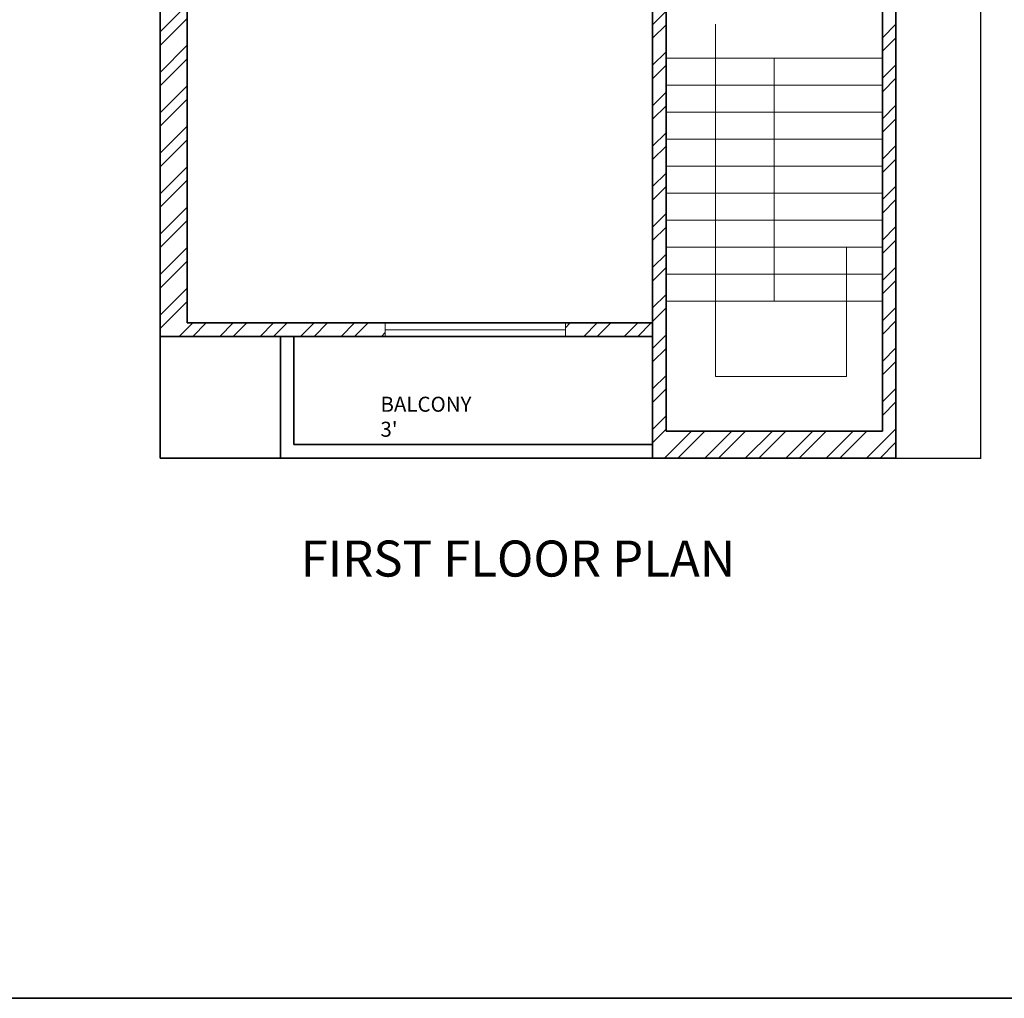
# Model space of a CAD drawing. Units: inches. Extents: x 1850 to 3445, y 1558 to 2756.
# Tile 5 of 13: x 2304 to 2632, y 1558 to 1884. Entities that reach past the tile are written whole.
import ezdxf

# ---------------------------------------------------------------- set-up
doc = ezdxf.new("R2010")
doc.units = ezdxf.units.IN
for name, color, linetype, lineweight in [('A-ANNO-DIMS', 2, 'Continuous', 18), ('A-ANNO-TEXT', 7, 'Continuous', 18), ('A-ANNO-TTLB', 7, 'Continuous', 35), ('A-AREA-IDEN', 7, 'Continuous', 18), ('A-FLOR-STRS', 7, 'Continuous', 18), ('A-GLAZ', 4, 'Continuous', 18), ('A-WALL', 7, 'Continuous', 35), ('A-WALL-PATT', 252, 'Continuous', 13)]:
    doc.layers.add(name, color=color, linetype=linetype, lineweight=lineweight)
doc.styles.get("Standard").update_dxf_attribs({"font": 'arial.ttf'})
doc.dimstyles.get("Standard").update_dxf_attribs({"dimtxt": 0.18, "dimasz": 0.18, "dimexe": 0.18, "dimexo": 0.0625, "dimgap": 0.09, "dimtad": 0, "dimtih": 1, "dimtoh": 1, "dimdec": 4, "dimzin": 0, "dimdsep": 46, "dimtxsty": 'Standard', "dimcen": 0.09, "dimadec": 0, "dimazin": 0, "dimtfac": 1, "dimtdec": 4, "dimtofl": 0, "dimtmove": 0, "dimatfit": 3, "dimfxl": 1, "dimtolj": 1, "dimtzin": 0, "dimarcsym": 0})

# ---------------------------------------------------------------- blocks, each defined once
blk = doc.blocks.new('WIN-60-W4_5')
for p, q in [((0, 60), (4.5, 60)), ((4.5, 60), (2.25, 60)), ((2.25, 60), (2.25, 0)), ((2.25, 0), (0, 0)), ((0, 0), (4.5, 0))]:
    blk.add_line(p, q)
blk = doc.blocks.new('STAIR-UPPER-FLIGHT')
for p, q in [((72, 81), (0, 81)), ((36, 0), (36, 81)), ((72, 72), (0, 72)), ((72, 63), (0, 63)), ((72, 54), (0, 54)), ((72, 45), (0, 45)), ((72, 36), (0, 36)), ((72, 27), (0, 27)), ((72, 18), (0, 18)), ((72, 9), (0, 9)), ((0, 0), (72, 0)), ((72, 0), (36, 0))]:
    blk.add_line(p, q)
blk = doc.blocks.new('*D83')
at = {"layer": 'A-ANNO-DIMS', "color": 0, "lineweight": -2, "transparency": 16777216}
for p, q in [((2596.12, 2216.18), (2624.49, 2216.18)), ((2624.31, 2216), (2624.31, 1977.12)), ((2624.31, 1737.86), (2624.31, 1976.75)), ((2596.12, 1737.68), (2624.49, 1737.68))]:
    blk.add_line(p, q, dxfattribs=at)
at = {"layer": 'A-ANNO-DIMS', "color": 0, "transparency": 16777216}
for points in [[(2624.28, 2216), (2624.34, 2216), (2624.31, 2216.18)], [(2624.28, 1737.86), (2624.34, 1737.86), (2624.31, 1737.68)]]:
    blk.add_solid(points, dxfattribs=at)
at = {"layer": 'Defpoints', "color": 0, "transparency": 16777216}
for p in [(2596.06, 2216.18), (2624.31, 2216.18), (2596.06, 1737.68)]:
    blk.add_point(p, dxfattribs=at)
at = {"layer": 'A-ANNO-DIMS', "color": 0, "transparency": 16777216, "insert": (2624.31, 1976.93), "char_height": 0.18, "attachment_point": 5}
blk.add_mtext('\\A1;478.5', dxfattribs=at)

msp = doc.modelspace()

# ---------------------------------------------------------------- hatches: boundary and pattern name
at = {"layer": 'A-WALL-PATT'}
h = msp.add_hatch(dxfattribs=at)
h.set_pattern_fill('ANSI32', color=256)
h.paths.add_polyline_path([(2519.5556, 1907.3936), (2523.9987, 1907.3936), (2523.9987, 1916.3936), (2519.5556, 1916.3936), (2515.0556, 1916.3936), (2510.5556, 1916.3936), (2510.5556, 1907.3936), (2515.0556, 1907.3936), (2515.0556, 1742.1843), (2515.0556, 1737.6843), (2596.0556, 1737.6843), (2596.0556, 1976.4962), (2591.5556, 1976.4962), (2591.5556, 1916.3936), (2561.2666, 1916.3936), (2561.2666, 1907.3936), (2591.5556, 1907.3936), (2591.5556, 1746.6843), (2519.5556, 1746.6843)])
h.paths.add_polyline_path([(2076.6481, 2211.6843), (2076.6481, 2216.1843), (2040.2715, 2216.1843), (2040.2715, 2175.83), (2044.7715, 2175.83), (2049.2715, 2175.83), (2049.2715, 2207.1843), (2076.6481, 2207.1843)])
h.paths.add_polyline_path([(2211.7715, 2216.1843), (2136.6481, 2216.1843), (2136.6481, 2207.1843), (2211.7715, 2207.1843)])
h.paths.add_polyline_path([(2285.2715, 2154.1843), (2250.6169, 2154.1843), (2250.6169, 2149.6843), (2280.7715, 2149.6843), (2280.7715, 2075.1843), (2236.3632, 2075.1843), (2236.3632, 2070.6843), (2285.2715, 2070.6843)])
h.paths.add_polyline_path([(2228.3485, 2154.1843), (2207.2715, 2154.1843), (2207.2715, 2075.1843), (2201.9819, 2075.1843), (2201.9819, 2070.6843), (2215.4663, 2070.6843), (2215.4663, 2072.9343), (2215.4663, 2075.1843), (2211.7715, 2075.1843), (2211.7715, 2149.6843), (2228.3485, 2149.6843)])
h.paths.add_polyline_path([(2049.2715, 2115.83), (2040.2715, 2115.83), (2040.2715, 2042.8465), (2049.2715, 2042.8465), (2049.2715, 2070.6843), (2168.6057, 2070.6843), (2168.6057, 2072.9343), (2168.6057, 2075.1843), (2049.2715, 2075.1843)])
h.paths.add_polyline_path([(2049.2715, 1982.8465), (2040.2715, 1982.8465), (2040.2715, 1910.2175), (2060.9481, 1910.2175), (2060.9481, 1914.7175), (2060.9481, 1919.2175), (2049.2715, 1919.2175)])
h.paths.add_polyline_path([(2132.4938, 1919.2175), (2108.9481, 1919.2175), (2108.9481, 1910.2175), (2132.4938, 1910.2175), (2132.4938, 1914.6749)])
h.paths.add_polyline_path([(2178.7715, 1938.6843), (2169.7715, 1938.6843), (2169.7715, 1919.2175), (2163.687, 1919.2175), (2163.687, 1910.2175), (2169.7715, 1910.2175), (2169.7715, 1854.6843), (2169.7715, 1845.6843), (2196.1287, 1845.6843), (2196.1287, 1850.1843), (2196.1287, 1854.6843), (2178.7715, 1854.6843)])
h.paths.add_polyline_path([(2049.2715, 1910.2175), (2040.2715, 1910.2175), (2040.2715, 1745.6843), (2049.2715, 1745.6843)])
h.paths.add_polyline_path([(2146.8861, 1766.7204), (2159.0894, 1766.7204), (2159.0894, 1777.0239), (2146.8861, 1777.0239)], flags=9)
h.paths.add_polyline_path([(2183.4664, 1798.4016), (2226.7338, 1798.4016), (2226.7338, 1817.0589), (2183.4664, 1817.0589)], flags=9)
h.paths.add_polyline_path([(2070.863, 1867.537), (2109.9796, 1867.537), (2109.9796, 1886.1943), (2070.863, 1886.1943)], flags=9)
h = msp.add_hatch(dxfattribs=at)
h.set_pattern_fill('ANSI32', color=256)
h.paths.add_polyline_path([(2403.5576, 2211.6843), (2403.5576, 2216.1843), (2351.0556, 2216.1843), (2351.0556, 2169.0079), (2360.0556, 2169.0079), (2360.0556, 2207.1843), (2403.5576, 2207.1843)])
h.paths.add_polyline_path([(2522.5556, 2216.1843), (2463.5576, 2216.1843), (2463.5576, 2207.1843), (2522.5556, 2207.1843)])
h.paths.add_polyline_path([(2596.0556, 2154.1843), (2562.6647, 2154.1843), (2562.6647, 2149.6843), (2591.5556, 2149.6843), (2591.5556, 2075.1843), (2522.5556, 2075.1843), (2522.5556, 2079.8699), (2518.0556, 2079.8699), (2518.0556, 2075.1843), (2511.9412, 2075.1843), (2511.9412, 2070.6843), (2591.5556, 2070.6843), (2591.5556, 2036.4962), (2596.0556, 2036.4962)])
h.paths.add_polyline_path([(2538.6647, 2154.1843), (2522.5556, 2154.1843), (2518.0556, 2154.1843), (2518.0556, 2102.7998), (2522.5556, 2102.7998), (2522.5556, 2149.6843), (2538.6647, 2149.6843)], flags=17)
h.paths.add_polyline_path([(2477.8689, 2072.9343), (2477.8689, 2075.1843), (2360.0556, 2075.1843), (2360.0556, 2109.0079), (2355.5556, 2109.0079), (2351.0556, 2109.0079), (2351.0556, 2043.8694), (2355.5556, 2043.8694), (2360.0556, 2043.8694), (2360.0556, 2070.6843), (2450.0556, 2070.6843), (2450.0556, 2045.0271), (2454.5556, 2045.0271), (2454.5556, 2070.6843), (2477.8689, 2070.6843)])
h.paths.add_polyline_path([(2360.0556, 2007.8694), (2351.0556, 2007.8694), (2351.0556, 1958.9131), (2355.5556, 1958.9131), (2360.0556, 1958.9131), (2360.0556, 1970.1843), (2450.0556, 1970.1843), (2450.0556, 1913.1843), (2443.7332, 1913.1843), (2443.7332, 1908.6843), (2454.5556, 1908.6843), (2454.5556, 1999.4184), (2450.0556, 1999.4184), (2450.0556, 1974.6843), (2360.0556, 1974.6843)])
h.paths.add_polyline_path([(2360.0556, 1908.6843), (2422.4247, 1908.6843), (2422.4247, 1910.9343), (2422.4247, 1913.1843), (2360.0556, 1913.1843), (2360.0556, 1934.9131), (2351.0556, 1934.9131), (2351.0556, 1778.1843), (2426.033, 1778.1843), (2426.033, 1780.4343), (2426.033, 1782.6843), (2360.0556, 1782.6843)])
h.paths.add_polyline_path([(2515.0556, 1782.6843), (2486.033, 1782.6843), (2486.033, 1778.1843), (2515.0556, 1778.1843)])

# ---------------------------------------------------------------- linework, layer by layer
at = {"layer": 'A-ANNO-TTLB'}
msp.add_lwpolyline([(1850.1793, 2756.3177), (3445.2682, 2756.3177), (3445.2682, 1557.7728), (1850.1793, 1557.7728)], close=True, dxfattribs=at)
at = {"layer": 'A-FLOR-STRS'}
for p, q in [((2536.0345, 1882.1893), (2536.0345, 1764.8415)), ((2579.6492, 1764.8415), (2579.6492, 1807.8818)), ((2536.0345, 1764.8415), (2579.6492, 1764.8415))]:
    msp.add_line(p, q, dxfattribs=at)
at = {"layer": 'A-WALL'}
for p, q in [((2351.0556, 2216.1843), (2351.0556, 1737.6843)), ((2596.0556, 2216.1843), (2596.0556, 1737.6843)), ((2360.0556, 1908.6843), (2360.0556, 1782.6843)), ((2515.0556, 1907.3936), (2515.0556, 1742.1843)), ((2519.5556, 1746.6843), (2519.5556, 1907.3936)), ((2591.5556, 1907.3936), (2591.5556, 1746.6843)), ((2360.0556, 1782.6843), (2515.0556, 1782.6843)), ((2351.0556, 1778.1843), (2515.0556, 1778.1843)), ((2391.1014, 1737.6843), (2391.1014, 1778.1843)), ((2395.6014, 1778.1843), (2395.6014, 1742.1843)), ((2591.5556, 1746.6843), (2519.5556, 1746.6843)), ((2395.6014, 1742.1843), (2515.0556, 1742.1843)), ((2515.0556, 1742.1843), (2515.0556, 1737.6843)), ((2351.0556, 1737.6843), (2596.0556, 1737.6843)), ((2395.6014, 1737.6843), (2391.1014, 1737.6843))]:
    msp.add_line(p, q, dxfattribs=at)

# ---------------------------------------------------------------- block references
at = {"layer": 'A-FLOR-STRS'}
msp.add_blockref('STAIR-UPPER-FLIGHT', (2519.556, 1789.882), dxfattribs=at)
at = {"layer": 'A-GLAZ', "extrusion": (0, 0, -1), "zscale": -1, "rotation": 90}
msp.add_blockref('WIN-60-W4_5', (-2426.033, 1778.1838), dxfattribs=at)

# ---------------------------------------------------------------- texts
at = {"layer": 'A-ANNO-TEXT', "insert": (2397.816, 1710.2138), "char_height": 12, "attachment_point": 1}
msp.add_mtext_dynamic_manual_height_columns('FIRST FLOOR PLAN ', width=206.199656, gutter_width=12.5, heights=[0], dxfattribs=at)
at = {"layer": 'A-AREA-IDEN', "insert": (2424.4199, 1758.1068), "char_height": 5, "attachment_point": 1}
msp.add_mtext_dynamic_manual_height_columns("BALCONY\\P3'", width=90.635672, gutter_width=12.5, heights=[0], dxfattribs=at)

# ---------------------------------------------------------------- dimensions: what is measured, and where the dimension line sits
at = {"layer": 'A-ANNO-DIMS'}
dim = msp.add_linear_dim(base=(2624.3056, 2216.1843), p1=(2596.0556, 1737.6843), p2=(2596.0556, 2216.1843), angle=90, dimstyle='Standard', override={"dimdec": 1, "dimlfac": 1, "dimrnd": 0, "dimzin": 0, "dimdsep": 46, "dimlunit": 2}, dxfattribs=at)
dim.commit()
dim.dimension.update_dxf_attribs({"geometry": '*D83', "text_midpoint": (2624.3056, 1976.9343)})

doc.saveas('drawing.dxf')
